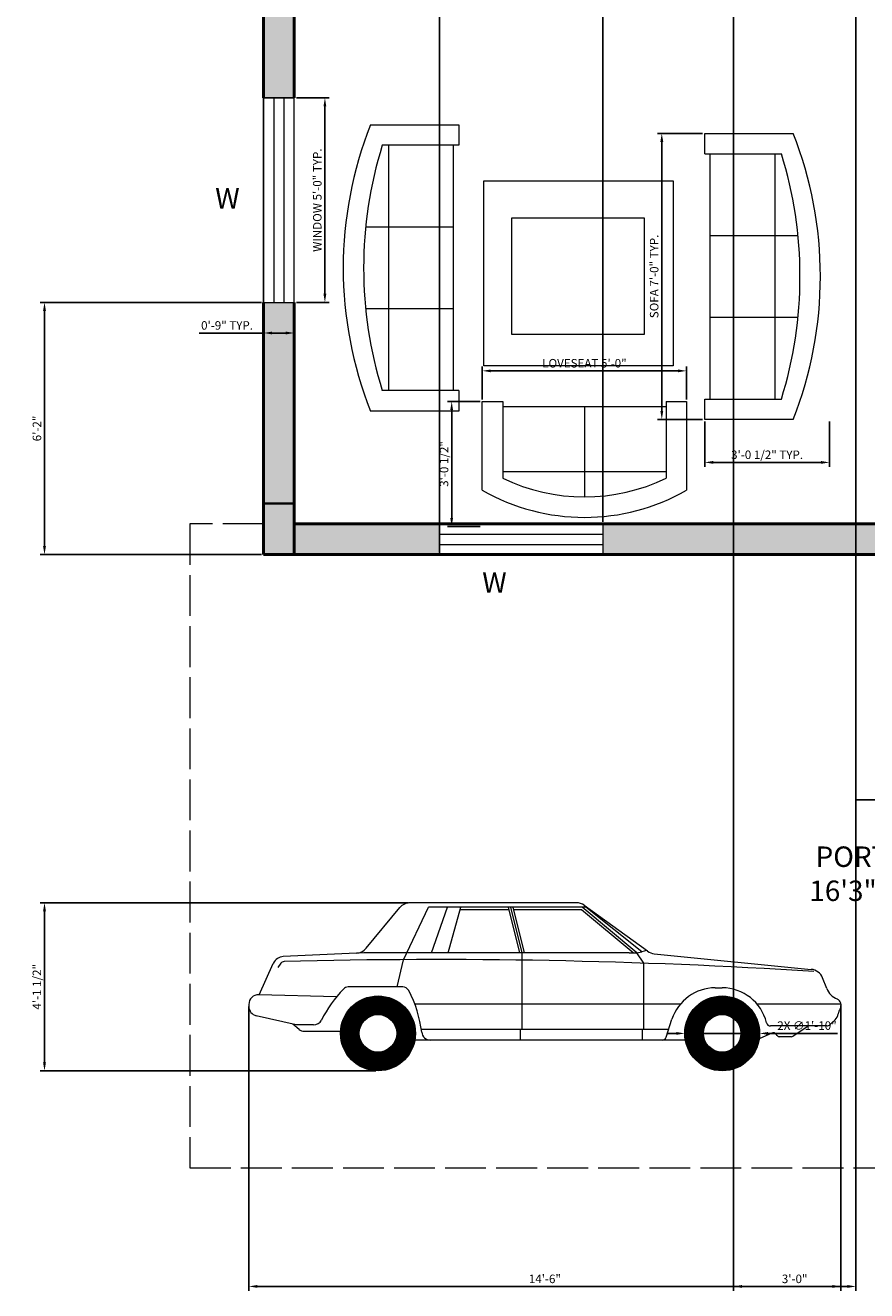
# Model space of a CAD drawing. Units: inches. Extents: x 5703 to 6226, y 10088 to 10813.
# Tile 1 of 5: x 5703 to 5950, y 10088 to 10460. Entities that reach past the tile are written whole.
import ezdxf

# ---------------------------------------------------------------- set-up
doc = ezdxf.new("R2010")
doc.units = ezdxf.units.IN
doc.linetypes.add('ACAD_ISO02W100', pattern=[15, 12, -3])
for name, color, linetype, lineweight in [('A-ANNO-DIMS', 2, 'Continuous', 18), ('A-ANNO-TEXT', 7, 'Continuous', 18), ('A-AREA-IDEN', 7, 'Continuous', 18), ('A-COLS', 7, 'Continuous', 35), ('A-COLS-PATT', 7, 'Continuous', 13), ('A-FLOR-STRS', 7, 'Continuous', 25), ('A-FURN', 8, 'Continuous', 18), ('A-SITE-VEHC', 8, 'Continuous', 18), ('A-WALL', 7, 'Continuous', 50), ('A-WALL-PATT', 9, 'Continuous', 13)]:
    doc.layers.add(name, color=color, linetype=linetype, lineweight=lineweight)
doc.layers.add('A-GLAZ', color=112, linetype='Continuous', lineweight=18, true_color=0x1ce368)
doc.layers.add('A-ROOF-OVHD', color=30, linetype='ACAD_ISO02W100', lineweight=18, true_color=0xf8991e)
doc.styles.get("Standard").update_dxf_attribs({"font": 'arial.ttf'})
doc.dimstyles.new('ISO-25', dxfattribs={"dimtxt": 2.5, "dimasz": 2.5, "dimexe": 1.25, "dimexo": 0.625, "dimtad": 1, "dimlunit": 3, "dimtxsty": 'Standard', "dimcen": 2.5, "dimadec": 0, "dimazin": 0, "dimtfac": 1, "dimtmove": 0, "dimatfit": 3, "dimfxl": 1, "dimarcsym": 0})

# ---------------------------------------------------------------- blocks, each defined once
blk = doc.blocks.new('Sofa - Roundback 7 ft.')
for p, q in [((-12.00002, -32.4421), (-12.00003, -6.5971)), ((11.99997, -32.4421), (11.99998, -6.5971)), ((-36.000027, -34), (-36.000027, -11.4696)), ((-35.999844, -13.3819), (35.9998, -13.3819)), ((35.99998, -34), (35.99998, -11.4696)), ((-36.000027, -32.4421), (35.99998, -32.4421))]:
    blk.add_line(p, q)
for points in [[(-36.000027, -34), (-42.000027, -34), (-42.000027, -8)], [(41.99998, -8), (41.99998, -34), (35.99998, -34)]]:
    blk.add_lwpolyline(points)
for centre, radius, start, end in [((0, -114.25), 114.25, 68.43141, 111.5686), ((-0.00001, -127.1968), 121.1968, 72.72033, 107.2797)]:
    blk.add_arc(centre, radius, start, end)
blk = doc.blocks.new('Sofa - Roundback Loveseat 5 ft.')
for p, q in [((0, -32.44198), (0, -5.99998)), ((-24, -33.99998), (-24, -11.46958)), ((-23.9998, -13.38178), (23.99986, -13.38178)), ((24.00004, -33.99998), (24.00004, -11.46958)), ((-24, -32.44198), (24.00004, -32.44198))]:
    blk.add_line(p, q)
for points in [[(-24, -33.99998), (-30, -33.99998), (-30, -7.99998)], [(30.00004, -7.99998), (30.00004, -33.99998), (24.00004, -33.99998)]]:
    blk.add_lwpolyline(points)
for centre, radius, start, end in [((0, -60.24998), 60.24998, 60.13715, 119.8628), ((0, -61.38438), 55.38444, 64.32083, 115.6792)]:
    blk.add_arc(centre, radius, start, end)
blk = doc.blocks.new('Car - sedan  side')
for p, q in [((-77.81, 49.34), (-126.58, 49.34)), ((-56.87, 35.13), (-75.48, 48.59)), ((-139.53, 35.99), (-129.64, 47.91)), ((-128.57, 32.64), (-121.22, 48.02)), ((-74.7, 48.02), (-121.22, 48.02)), ((-120.32, 34.67), (-115.67, 48.02)), ((-115.4, 34.67), (-111.74, 48.02)), ((-97.55, 47.3), (-111.94, 47.3)), ((-94.41, 34.67), (-97.73, 48.02)), ((-93.72, 34.67), (-97.04, 48.02)), ((-93.03, 34.67), (-96.34, 48.02)), ((-76.26, 47.3), (-96.16, 47.3)), ((-61.08, 34.66), (-76.26, 47.3)), ((-60.02, 34.65), (-76.07, 48.02)), ((-58.54, 34.93), (-74.99, 48.02)), ((-140.23, 34.67), (-163.88, 33.56)), ((-62.28, 34.67), (-140.23, 34.67)), ((-93.72, 19.62), (-93.72, 34.67)), ((-62.28, 34.67), (-60.02, 34.65)), ((-60.02, 34.65), (-58.54, 34.93)), ((-57.97, 31.61), (-60.02, 34.65)), ((-57.21, 35.38), (-58.54, 34.93)), ((-54.93, 34.4), (-8.75, 29.8)), ((-170.93, 22.32), (-166.81, 31.56)), ((-164.57, 31.6), (-165.48, 30.35)), ((-130.39, 24.63), (-128.57, 32.64)), ((-57.97, 19.62), (-57.97, 31.61)), ((-4.21, 24.18), (-5.42, 27.27)), ((-148.26, 21.7), (-171.11, 22.33)), ((-128.78, 24.63), (-144.79, 24.63)), ((-36.97, 24.38), (-34.94, 24.38)), ((-174, 19.51), (-174, 18.91)), ((-47.2, 19.62), (-125.23, 19.62)), ((-93.72, 12.14), (-93.72, 19.62)), ((-57.97, 12.14), (-57.97, 19.62)), ((0, 19.62), (-24.7, 19.62)), ((-160.12, 13.48), (-171.81, 16.16)), ((-51.4, 9.89), (-49.69, 15.14)), ((-3.22, 13.59), (-1.77, 14.97)), ((-159.22, 12.14), (-161.08, 13.7)), ((-155.01, 13.48), (-160.12, 13.48)), ((-147.03, 11.6), (-157.73, 11.6)), ((-50.67, 12.14), (-123.32, 12.14)), ((-94.21, 9.03), (-94.21, 12.14)), ((-58.39, 9.03), (-58.39, 12.14)), ((-4.23, 13.19), (-20.72, 13.19)), ((-9.5, 13.19), (-14.1, 10.2)), ((-120.62, 9.03), (-125.23, 9.03)), ((-45.76, 9.03), (-120.62, 9.03)), ((-20.36, 11.06), (-24.06, 9.44)), ((-18.83, 10.42), (-19.11, 10.76)), ((-14.68, 10.03), (-18.01, 10.03))]:
    blk.add_line(p, q)
at = {"const_width": 5.49}
for points in [[(-127.8, 11, -1), (-144.3, 11, -1)], [(-26.69, 11, -1), (-43.19, 11, -1)]]:
    blk.add_lwpolyline(points, format="xyb", close=True, dxfattribs=at)
for centre, radius in [((-136.05, 11), 11), ((-34.94, 11), 11), ((-136.05, 11), 5.51), ((-34.94, 11), 5.51)]:
    blk.add_circle(centre, radius)
for centre, radius, start, end in [((-126.58, 45.38), 3.97, 90, 140.3029), ((-77.81, 45.38), 3.97, 54.135, 90), ((-163.72, 30.18), 3.38, 92.6827, 155.9736), ((-142.58, 38.53), 3.97, 272.6827, 320.3029), ((-54.54, 38.35), 3.97, 234.135, 264.3123), ((-163.62, 30.91), 1.17, 91.491, 143.9553), ((-118.51, -1702.12), 1734.79, 86.34698, 91.49105), ((-9.15, 25.82), 4, 21.3107, 84.3123), ((-171.18, 19.51), 2.82, 88.4193, 180), ((-118.09, -2.78), 38.85, 136.3964, 152.9097), ((-144.79, 22.64), 1.98, 90, 136.3964), ((-128.78, 22.64), 1.98, 28.1371, 90), ((-157.14, 7.48), 34.14, 6.5135, 28.1371), ((-36.97, 11), 13.38, 90, 161.9732), ((-34.94, 11), 13.38, 13.5864, 90), ((0.9, 26.18), 5.49, 201.3107, 247.7048), ((-171.18, 18.91), 2.82, 180, 257.0905), ((-1.92, 19.3), 1.94, 325.3744, 67.7048), ((-155.01, 16.1), 2.62, 270, 332.9097), ((-3.82, 17.12), 2.96, 313.7173, 352.3839), ((2.46, 16.28), 3.37, 145.3744, 172.3839), ((-157.73, 13.93), 2.32, 230.1291, 270), ((-120.62, 11.65), 2.62, 186.5135, 270), ((-20.72, 14.43), 1.24, 193.5864, 270), ((-19.93, 10.09), 1.06, 39.301, 113.7159), ((-4.23, 14.65), 1.46, 270, 313.7173), ((-52.58, 10.27), 1.24, 270, 341.9732), ((-18.01, 11.09), 1.06, 219.301, 270), ((-14.68, 11.09), 1.06, 270, 303.047)]:
    blk.add_arc(centre, radius, start, end)
blk = doc.blocks.new('WIN-60x9')
for p, q in [((9, 60), (0, 60)), ((0, 60), (0, 0)), ((3, 60), (3, 0)), ((6, 0), (6, 60)), ((9, 0), (9, 60)), ((0, 0), (9, 0))]:
    blk.add_line(p, q)
blk = doc.blocks.new('*D16')
at = {"layer": 'A-ANNO-DIMS', "color": 0, "lineweight": -2, "transparency": 16777216}
for p, q in [((5902.12, 10428.04), (5888.9, 10428.04)), ((5890.15, 10425.54), (5890.15, 10346.54)), ((5902.12, 10344.04), (5888.9, 10344.04))]:
    blk.add_line(p, q, dxfattribs=at)
at = {"layer": 'A-ANNO-DIMS', "color": 0, "transparency": 16777216}
for points in [[(5889.73, 10425.54), (5890.57, 10425.54), (5890.15, 10428.04)], [(5889.73, 10346.54), (5890.57, 10346.54), (5890.15, 10344.04)]]:
    blk.add_solid(points, dxfattribs=at)
at = {"layer": 'Defpoints', "color": 0, "transparency": 16777216}
for p in [(5902.75, 10428.04), (5890.15, 10344.04), (5902.75, 10344.04)]:
    blk.add_point(p, dxfattribs=at)
at = {"layer": 'A-ANNO-DIMS', "color": 0, "transparency": 16777216, "insert": (5888.23, 10386.04), "char_height": 2.5, "attachment_point": 5, "rotation": 90}
blk.add_mtext('SOFA 7\'-0" TYP.', dxfattribs=at)
blk = doc.blocks.new('*D17')
at = {"layer": 'A-ANNO-DIMS', "color": 0, "lineweight": -2, "transparency": 16777216}
for p, q in [((5902.75, 10343.42), (5902.75, 10330.19)), ((5939.42, 10343.42), (5939.42, 10330.19)), ((5905.25, 10331.44), (5936.92, 10331.44))]:
    blk.add_line(p, q, dxfattribs=at)
at = {"layer": 'A-ANNO-DIMS', "color": 0, "transparency": 16777216}
for points in [[(5905.25, 10331.86), (5905.25, 10331.03), (5902.75, 10331.44)], [(5936.92, 10331.86), (5936.92, 10331.03), (5939.42, 10331.44)]]:
    blk.add_solid(points, dxfattribs=at)
at = {"layer": 'Defpoints', "color": 0, "transparency": 16777216}
for p in [(5902.75, 10344.04), (5939.42, 10344.04), (5939.42, 10331.44)]:
    blk.add_point(p, dxfattribs=at)
at = {"layer": 'A-ANNO-DIMS', "color": 0, "transparency": 16777216, "insert": (5921.08, 10333.36), "char_height": 2.5, "attachment_point": 5}
blk.add_mtext('3\'-0 1/2" TYP.', dxfattribs=at)
blk = doc.blocks.new('*D24')
at = {"layer": 'A-ANNO-DIMS', "color": 0, "lineweight": -2, "transparency": 16777216}
for p, q in [((5782.8, 10438.43), (5792.43, 10438.43)), ((5791.18, 10435.93), (5791.18, 10380.93)), ((5782.8, 10378.43), (5792.43, 10378.43))]:
    blk.add_line(p, q, dxfattribs=at)
at = {"layer": 'A-ANNO-DIMS', "color": 0, "transparency": 16777216}
for points in [[(5790.76, 10435.93), (5791.59, 10435.93), (5791.18, 10438.43)], [(5790.76, 10380.93), (5791.59, 10380.93), (5791.18, 10378.43)]]:
    blk.add_solid(points, dxfattribs=at)
at = {"layer": 'Defpoints', "color": 0, "transparency": 16777216}
for p in [(5782.18, 10438.43), (5782.18, 10378.43), (5791.18, 10378.43)]:
    blk.add_point(p, dxfattribs=at)
at = {"layer": 'A-ANNO-DIMS', "color": 0, "transparency": 16777216, "insert": (5789.26, 10408.43), "char_height": 2.5, "attachment_point": 5, "rotation": 90}
blk.add_mtext('WINDOW 5\'-0" TYP.', dxfattribs=at)
blk = doc.blocks.new('*D25')
at = {"layer": 'A-ANNO-DIMS', "color": 0, "lineweight": -2, "transparency": 16777216}
for p, q in [((5773.18, 10377.8), (5773.18, 10368.18)), ((5782.18, 10377.8), (5782.18, 10368.18)), ((5773.18, 10369.43), (5754.19, 10369.43)), ((5779.68, 10369.43), (5775.68, 10369.43))]:
    blk.add_line(p, q, dxfattribs=at)
at = {"layer": 'A-ANNO-DIMS', "color": 0, "transparency": 16777216}
for points in [[(5775.68, 10369.85), (5775.68, 10369.01), (5773.18, 10369.43)], [(5779.68, 10369.85), (5779.68, 10369.01), (5782.18, 10369.43)]]:
    blk.add_solid(points, dxfattribs=at)
at = {"layer": 'Defpoints', "color": 0, "transparency": 16777216}
for p in [(5773.18, 10378.43), (5782.18, 10378.43), (5773.18, 10369.43)]:
    blk.add_point(p, dxfattribs=at)
at = {"layer": 'A-ANNO-DIMS', "color": 0, "transparency": 16777216, "insert": (5762.43, 10371.33), "char_height": 2.5, "attachment_point": 5}
blk.add_mtext('0\'-9" TYP.', dxfattribs=at)
blk = doc.blocks.new('*D30')
at = {"layer": 'A-ANNO-DIMS', "color": 0, "lineweight": -2, "transparency": 16777216}
for p, q in [((5837.42, 10349.94), (5837.42, 10359.57)), ((5894.92, 10358.32), (5839.92, 10358.32)), ((5897.42, 10349.94), (5897.42, 10359.57))]:
    blk.add_line(p, q, dxfattribs=at)
at = {"layer": 'A-ANNO-DIMS', "color": 0, "transparency": 16777216}
for points in [[(5839.92, 10358.73), (5839.92, 10357.9), (5837.42, 10358.32)], [(5894.92, 10358.73), (5894.92, 10357.9), (5897.42, 10358.32)]]:
    blk.add_solid(points, dxfattribs=at)
at = {"layer": 'Defpoints', "color": 0, "transparency": 16777216}
for p in [(5837.42, 10358.32), (5837.42, 10349.32), (5897.42, 10349.32)]:
    blk.add_point(p, dxfattribs=at)
at = {"layer": 'A-ANNO-DIMS', "color": 0, "transparency": 16777216, "insert": (5867.42, 10360.23), "char_height": 2.5, "attachment_point": 5}
blk.add_mtext('LOVESEAT 5\'-0"', dxfattribs=at)
blk = doc.blocks.new('*D31')
at = {"layer": 'A-ANNO-DIMS', "color": 0, "lineweight": -2, "transparency": 16777216}
for p, q in [((5836.79, 10349.32), (5827.17, 10349.32)), ((5828.42, 10346.82), (5828.42, 10315.15)), ((5836.79, 10312.65), (5827.17, 10312.65))]:
    blk.add_line(p, q, dxfattribs=at)
at = {"layer": 'A-ANNO-DIMS', "color": 0, "transparency": 16777216}
for points in [[(5828, 10346.82), (5828.83, 10346.82), (5828.42, 10349.32)], [(5828, 10315.15), (5828.83, 10315.15), (5828.42, 10312.65)]]:
    blk.add_solid(points, dxfattribs=at)
at = {"layer": 'Defpoints', "color": 0, "transparency": 16777216}
for p in [(5837.42, 10349.32), (5828.42, 10312.65), (5837.42, 10312.65)]:
    blk.add_point(p, dxfattribs=at)
at = {"layer": 'A-ANNO-DIMS', "color": 0, "transparency": 16777216, "insert": (5826.5, 10330.98), "char_height": 2.5, "attachment_point": 5, "rotation": 90}
blk.add_mtext('3\'-0 1/2"', dxfattribs=at)
blk = doc.blocks.new('*D38')
at = {"layer": 'A-ANNO-DIMS', "color": 0, "lineweight": -2, "transparency": 16777216}
for p, q in [((5768.83, 10171.71), (5768.83, 10088.29)), ((5942.77, 10172.05), (5942.77, 10088.29)), ((5771.33, 10089.54), (5940.27, 10089.54))]:
    blk.add_line(p, q, dxfattribs=at)
at = {"layer": 'A-ANNO-DIMS', "color": 0, "transparency": 16777216}
for points in [[(5771.33, 10089.96), (5771.33, 10089.12), (5768.83, 10089.54)], [(5940.27, 10089.96), (5940.27, 10089.12), (5942.77, 10089.54)]]:
    blk.add_solid(points, dxfattribs=at)
at = {"layer": 'Defpoints', "color": 0, "transparency": 16777216}
for p in [(5768.83, 10172.34), (5942.77, 10172.67), (5942.77, 10089.54)]:
    blk.add_point(p, dxfattribs=at)
at = {"layer": 'A-ANNO-DIMS', "color": 0, "transparency": 16777216, "insert": (5855.8, 10091.44), "char_height": 2.5, "attachment_point": 5}
blk.add_mtext('14\'-6"', dxfattribs=at)
blk = doc.blocks.new('*D39')
at = {"layer": 'A-ANNO-DIMS', "color": 0, "lineweight": -2, "transparency": 16777216}
for p, q in [((5815.62, 10202.17), (5707.55, 10202.17)), ((5708.8, 10155.32), (5708.8, 10199.67)), ((5806.16, 10152.82), (5707.55, 10152.82))]:
    blk.add_line(p, q, dxfattribs=at)
at = {"layer": 'A-ANNO-DIMS', "color": 0, "transparency": 16777216}
for points in [[(5708.38, 10199.67), (5709.22, 10199.67), (5708.8, 10202.17)], [(5708.38, 10155.32), (5709.22, 10155.32), (5708.8, 10152.82)]]:
    blk.add_solid(points, dxfattribs=at)
at = {"layer": 'Defpoints', "color": 0, "transparency": 16777216}
for p in [(5708.8, 10202.17), (5816.25, 10202.17), (5806.78, 10152.82)]:
    blk.add_point(p, dxfattribs=at)
at = {"layer": 'A-ANNO-DIMS', "color": 0, "transparency": 16777216, "insert": (5706.88, 10177.5), "char_height": 2.5, "attachment_point": 5, "rotation": 90}
blk.add_mtext('4\'-1 1/2"', dxfattribs=at)
blk = doc.blocks.new('*D40')
at = {"layer": 'A-ANNO-DIMS', "color": 0, "lineweight": -2, "transparency": 16777216}
for p, q in [((5911.18, 10644.24), (5911.18, 10088.29)), ((5947.18, 10644.24), (5947.18, 10088.29)), ((5913.68, 10089.54), (5944.68, 10089.54))]:
    blk.add_line(p, q, dxfattribs=at)
at = {"layer": 'A-ANNO-DIMS', "color": 0, "transparency": 16777216}
for points in [[(5913.68, 10089.96), (5913.68, 10089.12), (5911.18, 10089.54)], [(5944.68, 10089.96), (5944.68, 10089.12), (5947.18, 10089.54)]]:
    blk.add_solid(points, dxfattribs=at)
at = {"layer": 'Defpoints', "color": 0, "transparency": 16777216}
for p in [(5911.18, 10644.87), (5947.18, 10644.87), (5947.18, 10089.54)]:
    blk.add_point(p, dxfattribs=at)
at = {"layer": 'A-ANNO-DIMS', "color": 0, "transparency": 16777216, "insert": (5929.18, 10091.44), "char_height": 2.5, "attachment_point": 5}
blk.add_mtext('3\'-0"', dxfattribs=at)
blk = doc.blocks.new('*D47')
at = {"layer": 'A-ANNO-DIMS', "color": 0, "lineweight": -2, "transparency": 16777216}
for p, q in [((5824.85, 10313.99), (5824.85, 10785.97)), ((5827.35, 10784.72), (5870.35, 10784.72)), ((5872.85, 10313.99), (5872.85, 10785.97))]:
    blk.add_line(p, q, dxfattribs=at)
at = {"layer": 'A-ANNO-DIMS', "color": 0, "transparency": 16777216}
for points in [[(5827.35, 10785.14), (5827.35, 10784.3), (5824.85, 10784.72)], [(5870.35, 10785.14), (5870.35, 10784.3), (5872.85, 10784.72)]]:
    blk.add_solid(points, dxfattribs=at)
at = {"layer": 'Defpoints', "color": 0, "transparency": 16777216}
for p in [(5872.85, 10784.72), (5824.85, 10313.37), (5872.85, 10313.37)]:
    blk.add_point(p, dxfattribs=at)
at = {"layer": 'A-ANNO-DIMS', "color": 0, "transparency": 16777216, "insert": (5848.85, 10786.62), "char_height": 2.5, "attachment_point": 5}
blk.add_mtext('4\'-0"', dxfattribs=at)
blk = doc.blocks.new('*D48')
at = {"layer": 'A-ANNO-DIMS', "color": 0, "lineweight": -2, "transparency": 16777216}
for p, q in [((5773.18, 10304.99), (5773.18, 10785.97)), ((5775.68, 10784.72), (5822.35, 10784.72)), ((5824.85, 10304.99), (5824.85, 10785.97))]:
    blk.add_line(p, q, dxfattribs=at)
at = {"layer": 'A-ANNO-DIMS', "color": 0, "transparency": 16777216}
for points in [[(5775.68, 10785.14), (5775.68, 10784.3), (5773.18, 10784.72)], [(5822.35, 10785.14), (5822.35, 10784.3), (5824.85, 10784.72)]]:
    blk.add_solid(points, dxfattribs=at)
at = {"layer": 'Defpoints', "color": 0, "transparency": 16777216}
for p in [(5824.85, 10784.72), (5773.18, 10304.37), (5824.85, 10304.37)]:
    blk.add_point(p, dxfattribs=at)
at = {"layer": 'A-ANNO-DIMS', "color": 0, "transparency": 16777216, "insert": (5799.01, 10786.64), "char_height": 2.5, "attachment_point": 5}
blk.add_mtext('4\'-3 1/2"', dxfattribs=at)
blk = doc.blocks.new('*D49')
at = {"layer": 'A-ANNO-DIMS', "color": 0, "lineweight": -2, "transparency": 16777216}
for p, q in [((5772.55, 10378.43), (5707.55, 10378.43)), ((5708.8, 10306.87), (5708.8, 10375.93)), ((5772.55, 10304.37), (5707.55, 10304.37))]:
    blk.add_line(p, q, dxfattribs=at)
at = {"layer": 'A-ANNO-DIMS', "color": 0, "transparency": 16777216}
for points in [[(5708.38, 10375.93), (5709.22, 10375.93), (5708.8, 10378.43)], [(5708.38, 10306.87), (5709.22, 10306.87), (5708.8, 10304.37)]]:
    blk.add_solid(points, dxfattribs=at)
at = {"layer": 'Defpoints', "color": 0, "transparency": 16777216}
for p in [(5708.8, 10378.43), (5773.18, 10378.43), (5773.18, 10304.37)]:
    blk.add_point(p, dxfattribs=at)
at = {"layer": 'A-ANNO-DIMS', "color": 0, "transparency": 16777216, "insert": (5706.9, 10341.4), "char_height": 2.5, "attachment_point": 5, "rotation": 90}
blk.add_mtext('6\'-2"', dxfattribs=at)
blk = doc.blocks.new('*D64')
at = {"layer": 'A-ANNO-DIMS', "color": 0, "lineweight": -2, "transparency": 16777216}
for p, q in [((5894.39, 10163.82), (5891.89, 10163.82)), ((5896.89, 10163.82), (5918.88, 10163.82)), ((5941.72, 10163.82), (5921.38, 10163.82))]:
    blk.add_line(p, q, dxfattribs=at)
at = {"layer": 'A-ANNO-DIMS', "color": 0, "transparency": 16777216}
for points in [[(5894.39, 10164.24), (5894.39, 10163.4), (5896.89, 10163.82)], [(5921.38, 10164.24), (5921.38, 10163.4), (5918.88, 10163.82)]]:
    blk.add_solid(points, dxfattribs=at)
at = {"layer": 'Defpoints', "color": 0, "transparency": 16777216}
for p in [(5896.89, 10163.82), (5918.88, 10163.82)]:
    blk.add_point(p, dxfattribs=at)
at = {"layer": 'A-ANNO-DIMS', "color": 0, "transparency": 16777216, "insert": (5932.8, 10165.79), "char_height": 2.5, "attachment_point": 5, "rotation": 359.9975}
blk.add_mtext('2X ∅1\'-10"', dxfattribs=at)

msp = doc.modelspace()

# ---------------------------------------------------------------- hatches: boundary and pattern name
at = {"layer": 'A-COLS-PATT'}
h = msp.add_hatch(color=256, dxfattribs=at)
h.dxf.hatch_style = 1
h.paths.add_polyline_path([(5788.176, 10725.869), (5773.176, 10725.869), (5773.176, 10716.869), (5788.176, 10716.869)])
h.paths.add_polyline_path([(5782.176, 10516.684), (5773.176, 10516.684), (5773.176, 10497.849), (5782.176, 10497.849)])
h.paths.add_polyline_path([(5782.176, 10319.369), (5773.176, 10319.369), (5773.176, 10304.369), (5782.176, 10304.369)])
h.paths.add_polyline_path([(5960.955, 10313.369), (5953.525, 10313.369), (5953.525, 10304.369), (5960.955, 10304.369)])
h.paths.add_polyline_path([(6040.176, 10314.869), (6031.176, 10314.869), (6031.176, 10304.369), (6040.176, 10304.369)])
h.paths.add_polyline_path([(6181.176, 10198.545), (6172.176, 10198.545), (6172.176, 10178.369), (6181.176, 10178.369)])
h.paths.add_polyline_path([(6181.176, 10505.369), (6172.176, 10505.369), (6172.176, 10492.633), (6181.176, 10492.633)])
h.paths.add_polyline_path([(6181.176, 10725.869), (6166.176, 10725.869), (6166.176, 10716.869), (6181.176, 10716.869)])
at = {"layer": 'A-WALL-PATT'}
h = msp.add_hatch(color=256, dxfattribs=at)
h.dxf.hatch_style = 1
h.paths.add_polyline_path([(6057.982, 10725.869), (6040.176, 10725.869), (6040.176, 10749.869), (5999.271, 10749.869), (5999.271, 10740.869), (6031.176, 10740.869), (6031.176, 10716.869), (6031.176, 10511.369), (6013.525, 10511.369), (6013.525, 10505.369), (6048.161, 10505.369), (6048.161, 10511.369), (6040.176, 10511.369), (6040.176, 10716.869), (6057.982, 10716.869)])
h.paths.add_polyline_path([(6166.176, 10725.869), (6093.982, 10725.869), (6093.982, 10716.869), (6166.176, 10716.869)])
h.paths.add_polyline_path([(6181.176, 10716.869), (6172.176, 10716.869), (6172.176, 10511.369), (6132.161, 10511.369, -0.0172363), (6132.161, 10509.369), (6132.161, 10505.369), (6181.176, 10505.369)])
h.paths.add_polyline_path([(6181.176, 10468.633), (6172.176, 10468.633), (6172.176, 10451.369), (6098.676, 10451.369), (6098.676, 10505.369), (6102.161, 10505.369), (6102.161, 10511.369), (6090.161, 10511.369), (6090.161, 10507.369, -0.0121933), (6090.161, 10505.369), (6092.676, 10505.369), (6092.676, 10451.369), (6085.668, 10451.369), (6085.668, 10445.369), (6092.676, 10445.369), (6172.176, 10445.369), (6172.176, 10342.529), (6181.176, 10342.529)])
h.paths.add_polyline_path([(6181.176, 10282.529), (6172.176, 10282.529), (6172.176, 10253.369), (6092.676, 10253.369), (6092.676, 10247.369), (6094.176, 10247.369), (6094.176, 10238.954), (6100.176, 10238.954), (6100.176, 10247.369), (6172.176, 10247.369), (6172.176, 10234.545), (6181.176, 10234.545)])
h.paths.add_polyline_path([(6172.176, 10187.369), (6100.176, 10187.369), (6100.176, 10220.954), (6096.176, 10220.954, -0.0293864), (6094.176, 10220.954), (6094.176, 10178.369), (6172.176, 10178.369)])
h.paths.add_polyline_path([(6050.745, 10187.369), (6040.176, 10187.369), (6040.176, 10178.369), (6050.745, 10178.369)])
h.paths.add_polyline_path([(6040.176, 10187.369), (6031.176, 10187.369), (6031.176, 10178.369), (6040.176, 10178.369)])
h.paths.add_polyline_path([(6040.176, 10304.369), (6031.176, 10304.369), (6031.176, 10187.369), (6040.176, 10187.369)])
h.paths.add_polyline_path([(6040.176, 10393.328), (6031.176, 10393.328), (6031.176, 10314.869), (6040.176, 10314.869)])
h.paths.add_polyline_path([(6040.176, 10445.369), (6046.458, 10445.369), (6046.458, 10451.369), (6031.176, 10451.369), (6031.176, 10408.328), (6040.176, 10408.328)])
h.paths.add_polyline_path([(5911.176, 10584.869), (5845.666, 10584.869, -0.0172363), (5845.666, 10582.869), (5845.666, 10578.869), (5902.176, 10578.869), (5902.176, 10505.369), (5953.525, 10505.369), (5953.525, 10511.369), (5911.176, 10511.369)])
h.paths.add_polyline_path([(5902.176, 10511.369), (5782.176, 10511.369), (5782.176, 10505.369), (5902.176, 10505.369)])
h.paths.add_polyline_path([(5782.176, 10578.869), (5815.666, 10578.869), (5815.666, 10584.869), (5773.176, 10584.869), (5773.176, 10516.684), (5782.176, 10516.684)])
h.paths.add_polyline_path([(5782.176, 10497.849), (5773.176, 10497.849), (5773.176, 10438.429), (5782.176, 10438.429)])
h.paths.add_polyline_path([(5782.176, 10378.429), (5773.176, 10378.429), (5773.176, 10319.369), (5782.176, 10319.369)])
h.paths.add_polyline_path([(5824.846, 10313.369), (5782.176, 10313.369), (5782.176, 10304.369), (5824.846, 10304.369)])
h.paths.add_polyline_path([(5953.525, 10313.369), (5872.846, 10313.369), (5872.846, 10304.369), (5953.525, 10304.369)])

# ---------------------------------------------------------------- linework, layer by layer
at = {"layer": 'A-COLS'}
for p, q in [((5782.176, 10319.369), (5773.176, 10319.369)), ((5782.176, 10304.369), (5782.176, 10319.369))]:
    msp.add_line(p, q, dxfattribs=at)
at = {"layer": 'A-FLOR-STRS'}
for q in [(5947.176, 10304.369), (5953.525, 10232.369)]:
    msp.add_line((5947.176, 10232.369), q, dxfattribs=at)
at = {"layer": 'A-FURN'}
for points in [[(5837.882, 10414.084), (5893.46, 10414.084), (5893.46, 10359.769), (5837.882, 10359.769)], [(5846.067, 10403.213), (5884.922, 10403.213), (5884.922, 10368.988), (5846.067, 10368.988)]]:
    msp.add_lwpolyline(points, close=True, dxfattribs=at)
at = {"layer": 'A-GLAZ'}
for p, q in [((5773.176, 10438.429), (5782.176, 10438.429)), ((5773.176, 10378.429), (5782.176, 10378.429)), ((5824.846, 10313.369), (5824.846, 10304.369)), ((5824.846, 10313.369), (5872.846, 10313.369)), ((5872.846, 10313.369), (5872.846, 10304.369)), ((5824.846, 10310.369), (5872.846, 10310.369)), ((5824.846, 10307.369), (5872.846, 10307.369)), ((5872.846, 10304.369), (5824.846, 10304.369))]:
    msp.add_line(p, q, dxfattribs=at)
at = {"layer": 'A-ROOF-OVHD'}
for p, q in [((5773.176, 10313.369), (5751.498, 10313.369)), ((5751.498, 10313.369), (5751.498, 10124.389)), ((5751.498, 10124.389), (6040.176, 10124.389))]:
    msp.add_line(p, q, dxfattribs=at)
at = {"layer": 'A-WALL'}
for p, q in [((5773.176, 10438.429), (5773.176, 10584.869)), ((5782.176, 10438.429), (5782.176, 10578.869)), ((5773.176, 10304.369), (5773.176, 10378.429)), ((5782.176, 10304.369), (5782.176, 10378.429)), ((5782.176, 10313.369), (5953.525, 10313.369)), ((5773.176, 10304.369), (5953.525, 10304.369))]:
    msp.add_line(p, q, dxfattribs=at)

# ---------------------------------------------------------------- block references
at = {"layer": 'A-FURN'}
for name, p, rotation in [('Sofa - Roundback 7 ft.', (5796.556, 10388.524), 89.99999999999999), ('Sofa - Roundback 7 ft.', (5936.749, 10386.042), 270), ('Sofa - Roundback Loveseat 5 ft.', (5867.418, 10315.316), 180)]:
    msp.add_blockref(name, p, dxfattribs=dict(at, rotation=rotation))
at = {"layer": 'A-GLAZ', "rotation": 180}
msp.add_blockref('WIN-60x9', (5782.177, 10438.429), dxfattribs=at)
at = {"layer": 'A-SITE-VEHC'}
msp.add_blockref('Car - sedan  side', (5942.827, 10152.824), dxfattribs=at)

# ---------------------------------------------------------------- texts
at = {"layer": 'A-ANNO-TEXT', "char_height": 6, "attachment_point": 1}
for insert in [(5757.116, 10411.965), (5835.561, 10299.179)]:
    msp.add_mtext_dynamic_manual_height_columns(' W', width=71.13425, gutter_width=12.5, heights=[0], dxfattribs=dict(at, insert=insert))
at = {"layer": 'A-AREA-IDEN', "insert": (5933.505, 10218.693), "char_height": 6, "attachment_point": 1}
msp.add_mtext_dynamic_manual_height_columns(' PORTICO\\P16\'3"X16\'0"', width=71.13425, gutter_width=12.5, heights=[0], dxfattribs=at)

# ---------------------------------------------------------------- dimensions: what is measured, and where the dimension line sits
at = {"layer": 'A-ANNO-DIMS'}
for base, p1, p2, picture, middle in [((5824.846, 10784.719), (5773.176, 10304.369), (5824.846, 10304.369), '*D48', (5799.011, 10786.637)), ((5872.846, 10784.719), (5824.846, 10313.369), (5872.846, 10313.369), '*D47', (5848.846, 10786.62)), ((5947.176, 10089.539), (5911.176, 10644.869), (5947.176, 10644.869), '*D40', (5929.176, 10091.442)), ((5942.774, 10089.539), (5768.827, 10172.338), (5942.774, 10172.674), '*D38', (5855.801, 10091.441))]:
    dim = msp.add_linear_dim(base=base, p1=p1, p2=p2, dimstyle='ISO-25', override={"dimdec": 1, "dimlfac": 1, "dimrnd": 0, "dimzin": 1, "dimdsep": 46, "dimlunit": 4, "dimfrac": 2}, dxfattribs=at)
    dim.commit()
    dim.dimension.update_dxf_attribs({"geometry": picture, "text_midpoint": middle})
for base, p1, p2, angle, text, picture, middle in [((5791.176, 10378.429), (5782.176, 10438.429), (5782.176, 10378.429), 270, 'WINDOW <> TYP.', '*D24', (5789.258, 10408.429)), ((5890.149, 10344.042), (5902.749, 10428.042), (5902.749, 10344.042), 270, 'SOFA <> TYP.', '*D16', (5888.23, 10386.042)), ((5773.176, 10369.429), (5782.176, 10378.429), (5773.176, 10378.429), 180, '<> TYP.', '*D25', (5762.432, 10371.331)), ((5837.418, 10358.316), (5897.418, 10349.316), (5837.418, 10349.316), 180, 'LOVESEAT <>', '*D30', (5867.418, 10360.234))]:
    dim = msp.add_linear_dim(base=base, p1=p1, p2=p2, angle=angle, text=text, dimstyle='ISO-25', override={"dimdec": 1, "dimlfac": 1, "dimrnd": 0, "dimzin": 1, "dimdsep": 46, "dimlunit": 4, "dimfrac": 2}, dxfattribs=at)
    dim.commit()
    dim.dimension.update_dxf_attribs({"geometry": picture, "text_midpoint": middle})
for base, p1, p2, angle, picture, middle in [((5708.799, 10378.429), (5773.176, 10304.369), (5773.176, 10378.429), 90, '*D49', (5706.897, 10341.399)), ((5828.418, 10312.649), (5837.418, 10349.316), (5837.418, 10312.649), 270, '*D31', (5826.499, 10330.983)), ((5708.799, 10202.169), (5806.78, 10152.824), (5816.246, 10202.169), 90, '*D39', (5706.881, 10177.497))]:
    dim = msp.add_linear_dim(base=base, p1=p1, p2=p2, angle=angle, dimstyle='ISO-25', override={"dimdec": 1, "dimlfac": 1, "dimrnd": 0, "dimzin": 1, "dimdsep": 46, "dimlunit": 4, "dimfrac": 2}, dxfattribs=at)
    dim.commit()
    dim.dimension.update_dxf_attribs({"geometry": picture, "text_midpoint": middle})
dim = msp.add_linear_dim(base=(5939.415, 10331.442), p1=(5902.749, 10344.042), p2=(5939.415, 10344.042), text='<> TYP.', dimstyle='ISO-25', override={"dimdec": 1, "dimlfac": 1, "dimrnd": 0, "dimzin": 1, "dimdsep": 46, "dimlunit": 4, "dimfrac": 2}, dxfattribs=at)
dim.commit()
dim.dimension.update_dxf_attribs({"geometry": '*D17', "text_midpoint": (5921.082, 10333.36)})
dim = msp.add_diameter_dim_2p(p1=(5896.89, 10163.821), p2=(5918.882, 10163.82), text='2X <>', dimstyle='ISO-25', override={"dimdec": 1, "dimlfac": 1, "dimrnd": 0, "dimzin": 1, "dimdsep": 46, "dimlunit": 4, "dimfrac": 2}, dxfattribs=at)
dim.commit()
dim.dimension.update_dxf_attribs({"geometry": '*D64', "text_midpoint": (5932.802, 10163.819)})

doc.saveas('drawing.dxf')
